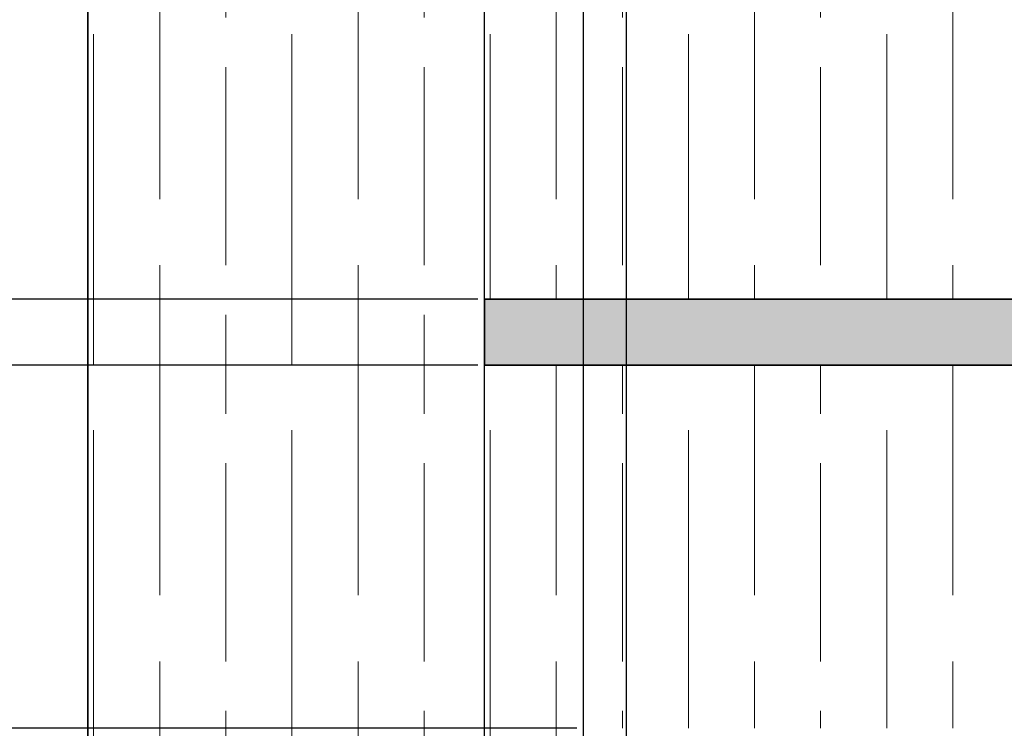
# Model space of a CAD drawing. Units: millimetres. Extents: x -692 to 9639, y -141 to 10345.
# Tile 14 of 19: x 3088 to 4578, y 8199 to 9272. Entities that reach past the tile are written whole.
import ezdxf

# ---------------------------------------------------------------- set-up
doc = ezdxf.new("R2010")
doc.units = ezdxf.units.MM
doc.header["$MEASUREMENT"] = 0
for name, color, linetype, lineweight in [('A-ANNO-DIMS', 2, 'Continuous', 18), ('A-ELEV', 7, 'Continuous', 35), ('A-ELEV-PATT', 8, 'Continuous', 13)]:
    doc.layers.add(name, color=color, linetype=linetype, lineweight=lineweight)
doc.styles.get("Standard").update_dxf_attribs({"font": 'arial.ttf'})
doc.dimstyles.get("Standard").update_dxf_attribs({"dimtxt": 25, "dimasz": 20, "dimexe": 0.18, "dimexo": 10, "dimgap": 10, "dimtad": 0, "dimtih": 1, "dimtoh": 1, "dimdec": 0, "dimzin": 0, "dimdsep": 46, "dimtxsty": 'Standard', "dimcen": 10, "dimadec": 0, "dimazin": 0, "dimtfac": 1, "dimtdec": 0, "dimtofl": 0, "dimtmove": 0, "dimatfit": 3, "dimfxl": 1, "dimtolj": 1, "dimtzin": 0, "dimarcsym": 0})

# ---------------------------------------------------------------- blocks, each defined once
blk = doc.blocks.new('*D7')
at = {"layer": 'A-ANNO-DIMS', "color": 0, "lineweight": -2, "transparency": 16777216}
for p, q in [((8481.5, 9848.8), (-649.1, 9848.8)), ((-648.9, 9828.8), (-648.9, 5124.9)), ((-648.9, 375.6), (-648.9, 5079.4)), ((2463.7, 355.6), (-649.1, 355.6))]:
    blk.add_line(p, q, dxfattribs=at)
at = {"layer": 'A-ANNO-DIMS', "color": 0, "lineweight": -3, "transparency": 16777216}
for points in [[(-652.2, 9828.8), (-645.6, 9828.8), (-648.9, 9848.8)], [(-652.2, 375.6), (-645.6, 375.6), (-648.9, 355.6)]]:
    blk.add_solid(points, dxfattribs=at)
at = {"layer": 'Defpoints', "color": 0, "lineweight": -3, "transparency": 16777216}
for p in [(-648.9, 9848.8), (8491.5, 9848.8), (2473.7, 355.6)]:
    blk.add_point(p, dxfattribs=at)
at = {"layer": 'A-ANNO-DIMS', "color": 0, "transparency": 16777216, "insert": (-648.9, 5102.2), "char_height": 25, "attachment_point": 5}
blk.add_mtext('\\A1;9493', dxfattribs=at)
blk = doc.blocks.new('*D52')
at = {"layer": 'A-ANNO-DIMS', "color": 0, "lineweight": -2, "transparency": 16777216}
for p, q in [((3791.5, 6858.8), (3791.5, 10329)), ((3811.5, 10328.8), (3830.1, 10328.8)), ((3921.5, 10328.8), (3902.9, 10328.8)), ((3941.5, 6708.8), (3941.5, 10329))]:
    blk.add_line(p, q, dxfattribs=at)
at = {"layer": 'A-ANNO-DIMS', "color": 0, "lineweight": -3, "transparency": 16777216}
for points in [[(3811.5, 10332.1), (3811.5, 10325.4), (3791.5, 10328.8)], [(3921.5, 10332.1), (3921.5, 10325.4), (3941.5, 10328.8)]]:
    blk.add_solid(points, dxfattribs=at)
at = {"layer": 'Defpoints', "color": 0, "lineweight": -3, "transparency": 16777216}
for p in [(3941.5, 10328.8), (3791.5, 6848.8), (3941.5, 6698.8)]:
    blk.add_point(p, dxfattribs=at)
at = {"layer": 'A-ANNO-DIMS', "color": 0, "transparency": 16777216, "insert": (3866.5, 10328.8), "char_height": 25, "attachment_point": 5}
blk.add_mtext('\\A1;150', dxfattribs=at)
blk = doc.blocks.new('*D53')
at = {"layer": 'A-ANNO-DIMS', "color": 0, "lineweight": -2, "transparency": 16777216}
for p, q in [((3941.5, 6708.8), (3941.5, 10329)), ((3961.5, 10328.8), (3986.3, 10328.8)), ((4006.3, 6433.8), (4006.3, 10329)), ((4006.3, 10328.8), (4026.3, 10328.8))]:
    blk.add_line(p, q, dxfattribs=at)
at = {"layer": 'A-ANNO-DIMS', "color": 0, "lineweight": -3, "transparency": 16777216}
for points in [[(3961.5, 10332.1), (3961.5, 10325.4), (3941.5, 10328.8)], [(3986.3, 10332.1), (3986.3, 10325.4), (4006.3, 10328.8)]]:
    blk.add_solid(points, dxfattribs=at)
at = {"layer": 'Defpoints', "color": 0, "lineweight": -3, "transparency": 16777216}
for p in [(4006.3, 10328.8), (3941.5, 6698.8), (4006.3, 6423.8)]:
    blk.add_point(p, dxfattribs=at)
at = {"layer": 'A-ANNO-DIMS', "color": 0, "transparency": 16777216, "insert": (4076.1, 10328.8), "char_height": 25, "attachment_point": 5}
blk.add_mtext('\\A1;64.71', dxfattribs=at)
blk = doc.blocks.new('*D54')
at = {"layer": 'A-ANNO-DIMS', "color": 0, "lineweight": -2, "transparency": 16777216}
for p, q in [((4006.3, 6433.8), (4006.3, 10329)), ((4026.3, 10328.8), (4497.5, 10328.8)), ((5061.3, 10328.8), (4590, 10328.8)), ((5081.3, 6433.8), (5081.3, 10329))]:
    blk.add_line(p, q, dxfattribs=at)
at = {"layer": 'A-ANNO-DIMS', "color": 0, "lineweight": -3, "transparency": 16777216}
for points in [[(4026.3, 10332.1), (4026.3, 10325.4), (4006.3, 10328.8)], [(5061.3, 10332.1), (5061.3, 10325.4), (5081.3, 10328.8)]]:
    blk.add_solid(points, dxfattribs=at)
at = {"layer": 'Defpoints', "color": 0, "lineweight": -3, "transparency": 16777216}
for p in [(5081.3, 10328.8), (4006.3, 6423.8), (5081.3, 6423.8)]:
    blk.add_point(p, dxfattribs=at)
at = {"layer": 'A-ANNO-DIMS', "color": 0, "transparency": 16777216, "insert": (4543.8, 10328.8), "char_height": 25, "attachment_point": 5}
blk.add_mtext('\\A1;1075', dxfattribs=at)
blk = doc.blocks.new('*D69')
at = {"layer": 'A-ANNO-DIMS', "color": 0, "lineweight": -2, "transparency": 16777216}
for p, q in [((3781.5, 8748.8), (-649.1, 8748.8)), ((-648.9, 8728.8), (-648.9, 8496.5)), ((-648.9, 8218.8), (-648.9, 8451)), ((3931.5, 8198.8), (-649.1, 8198.8))]:
    blk.add_line(p, q, dxfattribs=at)
at = {"layer": 'A-ANNO-DIMS', "color": 0, "lineweight": -3, "transparency": 16777216}
for points in [[(-652.2, 8728.8), (-645.6, 8728.8), (-648.9, 8748.8)], [(-652.2, 8218.8), (-645.6, 8218.8), (-648.9, 8198.8)]]:
    blk.add_solid(points, dxfattribs=at)
at = {"layer": 'Defpoints', "color": 0, "lineweight": -3, "transparency": 16777216}
for p in [(-648.9, 8748.8), (3791.5, 8748.8), (3941.5, 8198.8)]:
    blk.add_point(p, dxfattribs=at)
at = {"layer": 'A-ANNO-DIMS', "color": 0, "transparency": 16777216, "insert": (-648.9, 8473.8), "char_height": 25, "attachment_point": 5}
blk.add_mtext('\\A1;550', dxfattribs=at)
blk = doc.blocks.new('*D70')
at = {"layer": 'A-ANNO-DIMS', "color": 0, "lineweight": -2, "transparency": 16777216}
for p, q in [((-648.9, 8848.8), (-648.9, 8868.8)), ((-648.9, 8868.8), (-628.9, 8868.8)), ((3781.5, 8848.8), (-649.1, 8848.8)), ((-648.9, 8768.8), (-648.9, 8828.8)), ((3781.5, 8748.8), (-649.1, 8748.8))]:
    blk.add_line(p, q, dxfattribs=at)
at = {"layer": 'A-ANNO-DIMS', "color": 0, "lineweight": -3, "transparency": 16777216}
for points in [[(-652.2, 8828.8), (-645.6, 8828.8), (-648.9, 8848.8)], [(-652.2, 8768.8), (-645.6, 8768.8), (-648.9, 8748.8)]]:
    blk.add_solid(points, dxfattribs=at)
at = {"layer": 'Defpoints', "color": 0, "lineweight": -3, "transparency": 16777216}
for p in [(-648.9, 8848.8), (3791.5, 8848.8), (3791.5, 8748.8)]:
    blk.add_point(p, dxfattribs=at)
at = {"layer": 'A-ANNO-DIMS', "color": 0, "transparency": 16777216, "insert": (-592.5, 8868.8), "char_height": 25, "attachment_point": 5}
blk.add_mtext('\\A1;100', dxfattribs=at)

msp = doc.modelspace()

# ---------------------------------------------------------------- hatches: boundary and pattern name
at = {"layer": 'A-ELEV-PATT'}
h = msp.add_hatch(dxfattribs=at)
h.set_pattern_fill('GOST_WOOD', color=256, scale=50)
h.set_pattern_definition([(90, (0, 0), (300, -2e-14), [500, -100]), (90, (100, -100), (300, -2e-14), [300, -75, 150, -75]), (90, (200, -250), (300, -2e-14), [500, -100])])
edge = h.paths.add_edge_path()
edge.add_line((5191.547, 8748.772), (3791.547, 8748.772))
edge.add_line((3791.547, 8748.772), (3791.547, 8848.772))
edge.add_line((3791.547, 8848.772), (5191.547, 8848.772))
edge.add_line((5191.547, 8848.772), (5191.547, 9348.772))
edge.add_line((5191.547, 9348.772), (4755.992, 9348.772))
edge.add_line((4755.992, 9348.772), (4755.854, 9348.465))
edge.add_line((4755.854, 9348.465), (4755.734, 9348.772))
edge.add_line((4755.734, 9348.772), (4053.129, 9348.772))
edge.add_line((4053.129, 9348.772), (4052.99, 9348.465))
edge.add_line((4052.99, 9348.465), (4052.871, 9348.772))
edge.add_line((4052.871, 9348.772), (3701.731, 9348.772))
edge.add_line((3701.731, 9348.772), (3701.593, 9348.465))
edge.add_line((3701.593, 9348.465), (3701.474, 9348.772))
edge.add_line((3701.474, 9348.772), (3368.199, 9348.772))
edge.add_line((3368.199, 9348.772), (3368.061, 9348.465))
edge.add_line((3368.061, 9348.465), (3367.942, 9348.772))
edge.add_line((3367.942, 9348.772), (3191.547, 9348.772))
edge.add_line((3191.547, 9348.772), (3191.547, 3210.058))
edge.add_spline(control_points=[(3191.547, 3210.058), (3198.467, 3207.5), (3283.859, 3166.656), (3324.053, 2995.08), (3234.02, 2920.058), (3220.783, 2911.684)], knot_values=[13649.89756952, 13649.89756952, 13649.89756952, 13649.89756952, 13672.14990348, 13935.42377748, 13974.4426778, 13974.4426778, 13974.4426778, 13974.4426778], degree=3, periodic=0)
edge.add_spline(control_points=[(3220.783, 2911.684), (3225.148, 2890.107), (3226.864, 2868.931), (3226.144, 2848.27)], knot_values=[8828.69997321, 8828.69997321, 8828.69997321, 8828.69997321, 8890.6429847, 8890.6429847, 8890.6429847, 8890.6429847], degree=3, periodic=0)
edge.add_line((3226.144, 2848.27), (5191.547, 2848.27))
edge.add_line((5191.547, 2848.27), (5191.547, 3048.27))
edge.add_line((5191.547, 3048.27), (5041.547, 3048.27))
edge.add_line((5041.547, 3048.27), (5041.547, 3148.27))
edge.add_line((5041.547, 3148.27), (5091.547, 3148.27))
edge.add_line((5091.547, 3148.27), (5091.547, 3598.27))
edge.add_line((5091.547, 3598.27), (5191.547, 3598.27))
edge.add_line((5191.547, 3598.27), (5191.547, 4848.772))
edge.add_line((5191.547, 4848.772), (3791.547, 4848.772))
edge.add_line((3791.547, 4848.772), (3791.547, 6848.772))
edge.add_line((3791.547, 6848.772), (5091.547, 6848.772))
edge.add_line((5091.547, 6848.772), (5091.547, 7298.772))
edge.add_line((5091.547, 7298.772), (5191.547, 7298.772))
edge.add_line((5191.547, 7298.772), (5191.547, 8748.772))
h.paths.add_polyline_path([(5016.547, 8198.772), (5016.547, 7123.772), (3941.547, 7123.772), (3941.547, 8198.772)], flags=16)
h.paths.add_polyline_path([(4941.547, 8123.772), (4941.547, 7198.772), (4016.547, 7198.772), (4016.547, 8123.772)], flags=0)
h.paths.add_polyline_path([(4616.547, 8073.772), (4616.547, 7248.772), (4341.547, 7248.772), (4341.547, 8073.772)], flags=0)
h.paths.add_polyline_path([(4641.547, 8073.772), (4891.547, 8073.772), (4891.547, 7248.772), (4641.547, 7248.772)], flags=0)
h.paths.add_polyline_path([(4666.547, 8048.772), (4866.547, 8048.772), (4866.547, 7273.772), (4666.547, 7273.772)], flags=0)
h.paths.add_polyline_path([(4316.547, 8073.772), (4316.547, 7248.772), (4066.547, 7248.772), (4066.547, 8073.772)], flags=0)
h.paths.add_polyline_path([(4291.547, 8048.772), (4291.547, 7273.772), (4091.547, 7273.772), (4091.547, 8048.772)], flags=0)
h.paths.add_polyline_path([(5016.547, 4497.772), (5016.547, 3422.772), (3941.547, 3422.772), (3941.547, 4497.772)], flags=16)
h.paths.add_polyline_path([(4941.547, 4422.772), (4941.547, 3497.772), (4016.547, 3497.772), (4016.547, 4422.772)], flags=0)
h.paths.add_polyline_path([(4616.547, 4372.772), (4616.547, 3547.772), (4341.547, 3547.772), (4341.547, 4372.772)], flags=0)
h.paths.add_polyline_path([(4641.547, 4372.772), (4891.547, 4372.772), (4891.547, 3547.772), (4641.547, 3547.772)], flags=0)
h.paths.add_polyline_path([(4316.547, 4372.772), (4316.547, 3547.772), (4066.547, 3547.772), (4066.547, 4372.772)], flags=0)
h.paths.add_polyline_path([(4666.547, 4347.772), (4866.547, 4347.772), (4866.547, 3572.772), (4666.547, 3572.772)], flags=0)
h.paths.add_polyline_path([(4291.547, 4347.772), (4291.547, 3572.772), (4091.547, 3572.772), (4091.547, 4347.772)], flags=0)
h = msp.add_hatch(dxfattribs=at)
h.set_pattern_fill('CROSS', color=256, scale=150)
h.paths.add_polyline_path([(8491.547, 8848.772), (3791.547, 8848.772), (3791.547, 8748.772), (8391.547, 8748.772), (8391.547, 6848.772), (8491.547, 6848.772)])

# ---------------------------------------------------------------- linework, layer by layer
at = {"layer": 'A-ELEV'}
for p, q in [((3191.547, 2848.27), (3191.547, 9348.772)), ((3791.547, 8848.772), (8491.547, 8848.772)), ((3791.547, 8748.772), (3791.547, 8848.772)), ((3791.547, 8748.772), (8391.547, 8748.772))]:
    msp.add_line(p, q, dxfattribs=at)

# ---------------------------------------------------------------- dimensions: what is measured, and where the dimension line sits
at = {"layer": 'A-ANNO-DIMS'}
for base, p1, p2, override, picture, middle in [((3941.547, 10328.772), (3791.547, 6848.772), (3941.547, 6698.772), {"dimdec": 0, "dimlfac": 1, "dimrnd": 0, "dimzin": 0, "dimdsep": 46, "dimlunit": 2}, '*D52', (3866.547, 10328.772)), ((4006.259, 10328.772), (3941.547, 6698.772), (4006.259, 6423.772), {"dimdec": 2, "dimlfac": 1, "dimrnd": 0, "dimzin": 0, "dimdsep": 46, "dimlunit": 2}, '*D53', (4076.095, 10328.772)), ((5081.259, 10328.772), (4006.259, 6423.772), (5081.259, 6423.772), {"dimdec": 0, "dimlfac": 1, "dimrnd": 0, "dimzin": 0, "dimdsep": 46, "dimlunit": 2}, '*D54', (4543.759, 10328.772))]:
    dim = msp.add_linear_dim(base=base, p1=p1, p2=p2, dimstyle='Standard', override=override, dxfattribs=at)
    dim.commit()
    dim.dimension.update_dxf_attribs({"geometry": picture, "text_midpoint": middle})
for base, p1, p2, picture, middle in [((-648.912, 9848.772), (2473.746, 355.575), (8491.547, 9848.772), '*D7', (-648.912, 5102.173)), ((-648.912, 8848.772), (3791.547, 8748.772), (3791.547, 8848.772), '*D70', (-592.514, 8868.772)), ((-648.912, 8748.772), (3941.547, 8198.772), (3791.547, 8748.772), '*D69', (-648.912, 8473.772))]:
    dim = msp.add_linear_dim(base=base, p1=p1, p2=p2, angle=90, dimstyle='Standard', override={"dimdec": 0, "dimlfac": 1, "dimrnd": 0, "dimzin": 0, "dimdsep": 46, "dimlunit": 2}, dxfattribs=at)
    dim.commit()
    dim.dimension.update_dxf_attribs({"geometry": picture, "text_midpoint": middle})

doc.saveas('drawing.dxf')
